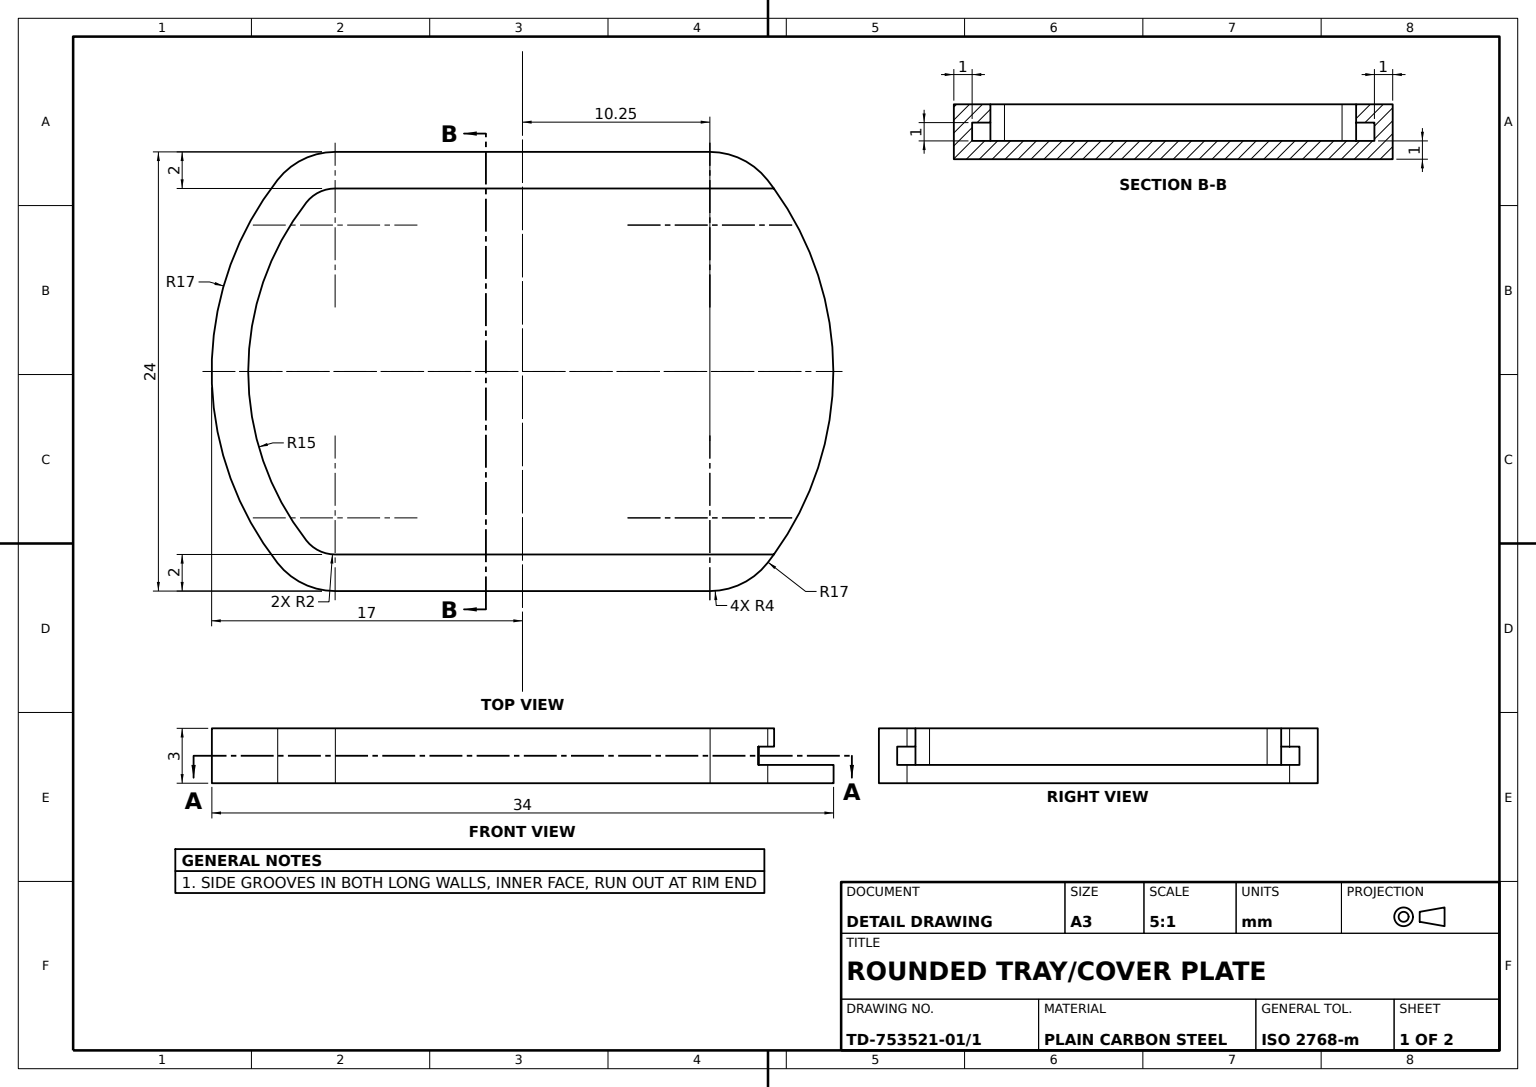
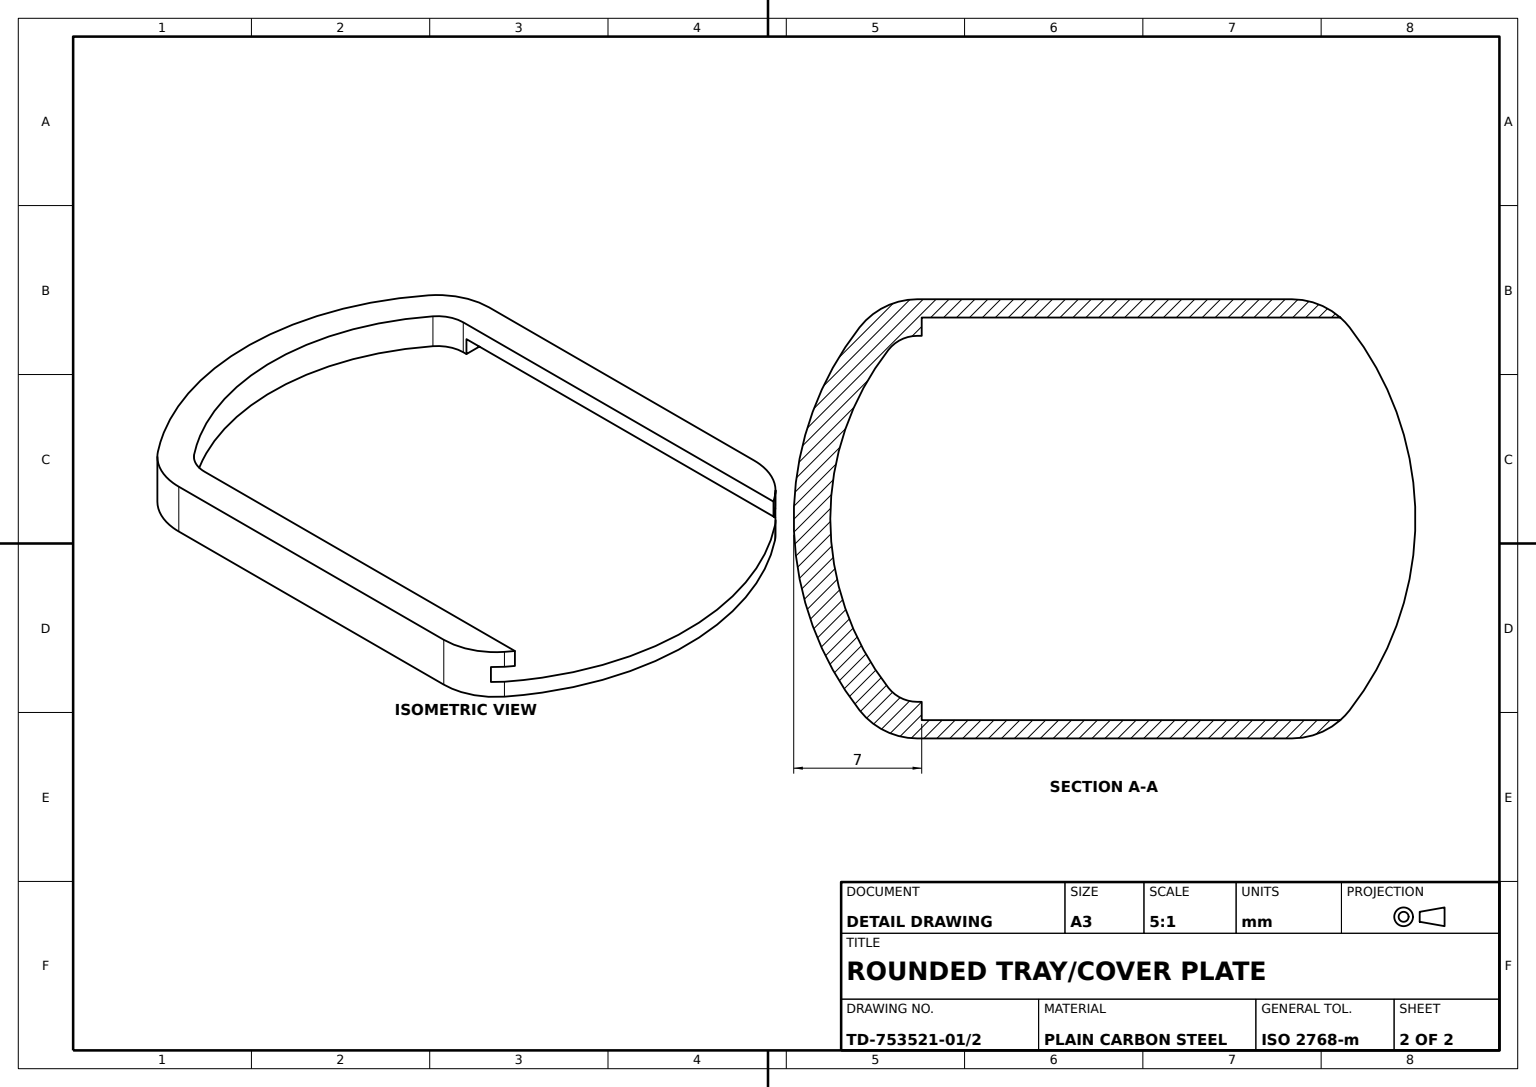
from build123d import *

# Parameters (mm, degrees)
BASE_PLATE_DEPTH       = 1
RIM_WALL_DEPTH         = 2
SIDE_GROOVE_A_SKETCH_W = 1
SIDE_GROOVE_A_SKETCH_H = 1
SIDE_GROOVE_A_DEPTH    = 40
SIDE_GROOVE_B_SKETCH_W = 1
SIDE_GROOVE_B_SKETCH_H = 1
SIDE_GROOVE_B_DEPTH    = 40


with BuildPart() as part:
    # Base Plate Sketch → Base Plate (new body)
    with BuildSketch(Plane(origin=(0, 0, 0), x_dir=(1, 0, 0), z_dir=(0, 1, 0))):
        with BuildLine():
            Line((-10.246950766, 12), (10.246950766, 12))
            ThreePointArc((10.246950766, 12), (12.001066805, 11.594868137), (13.399858694, 10.461538462))
            ThreePointArc((13.399858694, 10.461538462), (17, 0), (13.399858694, -10.461538462))
            ThreePointArc((13.399858694, -10.461538462), (12.001066805, -11.594868137), (10.246950766, -12))
            Line((10.246950766, -12), (-10.246950766, -12))
            ThreePointArc((-10.246950766, -12), (-12.001066805, -11.594868137), (-13.399858694, -10.461538462))
            ThreePointArc((-13.399858694, -10.461538462), (-17, 0), (-13.399858694, 10.461538462))
            ThreePointArc((-13.399858694, 10.461538462), (-12.001066805, 11.594868137), (-10.246950766, 12))
        make_face()
    extrude(amount=BASE_PLATE_DEPTH)

    # Rim Wall Sketch → Rim Wall (add)
    with BuildSketch(Plane(origin=(0, 1, 0), x_dir=(1, 0, 0), z_dir=(0, 1, 0))):
        with BuildLine():
            Line((10.246950766, -10), (-10.246950766, -10))
            ThreePointArc((-10.246950766, -10), (-11.124008785, -9.797434069), (-11.82340473, -9.230769231))
            ThreePointArc((-11.82340473, -9.230769231), (-15, 0), (-11.82340473, 9.230769231))
            ThreePointArc((-11.82340473, 9.230769231), (-11.124008785, 9.797434069), (-10.246950766, 10))
            Line((-10.246950766, 10), (10.246950766, 10))
            Line((10.246950766, 10), (13.747727085, 10))
            ThreePointArc((13.747727085, 10), (13.575754412, 10.232247659), (13.399858694, 10.461538462))
            ThreePointArc((13.399858694, 10.461538462), (12.001066805, 11.594868137), (10.246950766, 12))
            Line((10.246950766, 12), (-10.246950766, 12))
            ThreePointArc((-10.246950766, 12), (-12.001066805, 11.594868137), (-13.399858694, 10.461538462))
            ThreePointArc((-13.399858694, 10.461538462), (-17, 0), (-13.399858694, -10.461538462))
            ThreePointArc((-13.399858694, -10.461538462), (-12.001066805, -11.594868137), (-10.246950766, -12))
            Line((-10.246950766, -12), (10.246950766, -12))
            ThreePointArc((10.246950766, -12), (12.001066805, -11.594868137), (13.399858694, -10.461538462))
            ThreePointArc((13.399858694, -10.461538462), (13.575754412, -10.232247659), (13.747727085, -10))
            Line((13.747727085, -10), (10.246950766, -10))
        make_face()
    extrude(amount=RIM_WALL_DEPTH)

    # Side Groove A Sketch → Side Groove A (cut)
    with BuildSketch(Plane(origin=(30, 0, 0), x_dir=(0, 0, -1), z_dir=(1, 0, 0))):
        with Locations((-10.5, 1.5)):
            Rectangle(SIDE_GROOVE_A_SKETCH_W, SIDE_GROOVE_A_SKETCH_H)
    extrude(amount=-SIDE_GROOVE_A_DEPTH, mode=Mode.SUBTRACT)

    # Side Groove B Sketch → Side Groove B (cut)
    with BuildSketch(Plane(origin=(30, 0, 0), x_dir=(0, 0, -1), z_dir=(1, 0, 0))):
        with Locations((10.5, 1.5)):
            Rectangle(SIDE_GROOVE_B_SKETCH_W, SIDE_GROOVE_B_SKETCH_H)
    extrude(amount=-SIDE_GROOVE_B_DEPTH, mode=Mode.SUBTRACT)


solid = part.part
